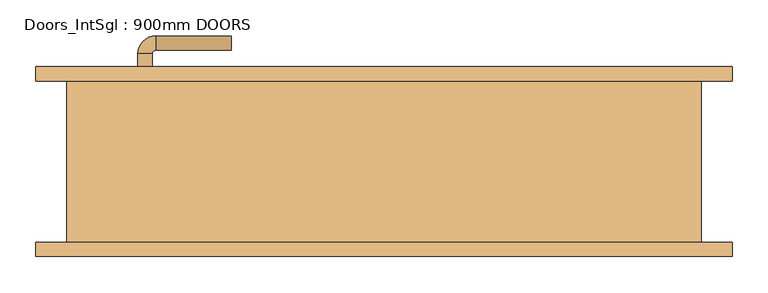
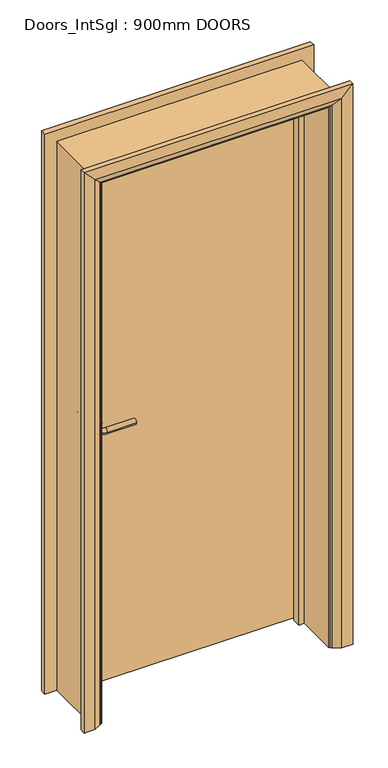
"""IFC4 building model written with IfcOpenShell, lengths in millimetres: door geometry, Doors_IntSgl : 900mm DOORS."""

from ifc_helpers import new_model, si_unit, point, frame, frame_2d, origin, place, context, project, spatial, polyline, circle_curve, ellipse_curve, trimmed, segment, composite_curve, outline, extrude, faceted_brep, source, transform, mapped, element, save
from ifc_brep_helpers import plane_surface, cylinder_surface, revolved_surface, advanced_brep


def doors_intsgl_900mm_doors_1c9cf9a6(model_context):
    return source(origin(), model_context, "Body", "SolidModel", [
        advanced_brep(
        [(-343.0, 66.5, 1000.0), (-323.0, 66.5, 1000.0), (-323.0, 36.5, 1000.0), (-343.0, 36.5, 1000.0), (-318.0, 31.5, 1000.0), (-318.0, 11.5, 1000.0), (-213.0, 11.5, 1000.0), (-213.0, 31.5, 1000.0)],
        [
            (0, 1, circle_curve(frame((-333.0, 66.5, 1000.0), z_axis=(0.0, 1.0, 0.0), x_axis=(1.0, 0.0, 0.0)), 10.0)),
            (1, 0, circle_curve(frame((-333.0, 66.5, 1000.0), z_axis=(0.0, 1.0, 0.0), x_axis=(1.0, 0.0, 0.0)), 10.0)),
            (1, 2),
            (2, 3, circle_curve(frame((-333.0, 36.5, 1000.0), z_axis=(0.0, 1.0, 0.0), x_axis=(1.0, 0.0, 0.0)), 10.0)),
            (3, 0),
            (3, 2, circle_curve(frame((-333.0, 36.5, 1000.0), z_axis=(0.0, 1.0, 0.0), x_axis=(1.0, 0.0, 0.0)), 10.0)),
            (4, 5, circle_curve(frame((-318.0, 21.5, 1000.0), z_axis=(-1.0, 0.0, 0.0), x_axis=(0.0, 1.0, 0.0)), 10.0)),
            (5, 3, circle_curve(frame((-318.0, 36.5, 1000.0), z_axis=(0.0, 0.0, -1.0), x_axis=(-1.0, 0.0, 0.0)), 25.0)),
            (2, 4, circle_curve(frame((-318.0, 36.5, 1000.0), z_axis=(0.0, 0.0, 1.0), x_axis=(-1.0, 0.0, 0.0)), 5.0)),
            (5, 4, circle_curve(frame((-318.0, 21.5, 1000.0), z_axis=(-1.0, 0.0, 0.0), x_axis=(0.0, 1.0, 0.0)), 10.0)),
            (6, 7, circle_curve(frame((-213.0, 21.5, 1000.0), z_axis=(1.0, 0.0, 0.0), x_axis=(0.0, 1.0, 0.0)), 10.0)),
            (7, 6, circle_curve(frame((-213.0, 21.5, 1000.0), z_axis=(1.0, 0.0, 0.0), x_axis=(0.0, 1.0, 0.0)), 10.0)),
            (4, 7),
            (6, 5),
        ],
        [
            plane_surface(frame((-333.0, 66.5, 1000.0), z_axis=(0.0, 1.0, 0.0), x_axis=(0.0, 0.0, 1.0))),
            cylinder_surface(frame((-333.0, 66.5, 1000.0), z_axis=(0.0, 1.0, 0.0), x_axis=(1.0, 0.0, 0.0)), 10.0),
            revolved_surface(trimmed(ellipse_curve(frame((-333.0, 36.5, 1000.0), z_axis=(0.0, -1.0, 0.0), x_axis=(1.0, 0.0, 0.0)), 10.0, 10.0), [point((-343.0, 36.5, 1000.0))], [point((-323.0, 36.5, 1000.0))], True, "CARTESIAN"), (-318.0, 36.5, 1000.0), (0.0, 0.0, -1.0)),
            revolved_surface(trimmed(ellipse_curve(frame((-333.0, 36.5, 1000.0), z_axis=(0.0, -1.0, 0.0), x_axis=(1.0, 0.0, 0.0)), 10.0, 10.0), [point((-323.0, 36.5, 1000.0))], [point((-343.0, 36.5, 1000.0))], True, "CARTESIAN"), (-318.0, 36.5, 1000.0), (0.0, 0.0, -1.0)),
            plane_surface(frame((-213.0, 21.5, 1000.0), z_axis=(1.0, 0.0, 0.0), x_axis=(0.0, 0.0, 1.0))),
            cylinder_surface(frame((-318.0, 21.5, 1000.0), z_axis=(-1.0, 0.0, 0.0), x_axis=(0.0, 1.0, 0.0)), 10.0),
        ],
        [
            (0, [[1, 2]]),
            (1, [[3, 4, 5, -2]]),
            (1, [[-5, 6, -3, -1]]),
            (2, [[7, 8, -4, 9]]),
            (3, [[10, -9, -6, -8]]),
            (4, [[11, 12]]),
            (5, [[13, -11, 14, -7]]),
            (5, [[-14, -12, -13, -10]]),
        ],
    ),
        extrude(outline(composite_curve([segment(trimmed(circle_curve(frame_2d((1000.0, -335.5)), 30.0), [point((1000.0, -365.5))], [point((1000.0, -305.5))], False, "CARTESIAN"), True, "CONTINUOUS"), segment(trimmed(circle_curve(frame_2d((1000.0, -335.5)), 30.0), [point((1000.0, -305.5))], [point((1000.0, -365.5))], False, "CARTESIAN"), True, "CONTINUOUS")], self_intersect=False)), frame((0.0, 66.5, 0.0), z_axis=(0.0, 1.0, 0.0), x_axis=(0.0, 0.0, 1.0)), (0.0, 0.0, 1.0), 8.0),
        advanced_brep(
        [(-343.0, 120.5, 1000.0), (-323.0, 120.5, 1000.0), (-343.0, 150.5, 1000.0), (-323.0, 150.5, 1000.0), (-318.0, 155.5, 1000.0), (-318.0, 175.5, 1000.0), (-213.0, 175.5, 1000.0), (-213.0, 155.5, 1000.0)],
        [
            (0, 1, circle_curve(frame((-333.0, 120.5, 1000.0), z_axis=(0.0, -1.0, 0.0), x_axis=(1.0, 0.0, 0.0)), 10.0)),
            (1, 0, circle_curve(frame((-333.0, 120.5, 1000.0), z_axis=(0.0, -1.0, 0.0), x_axis=(1.0, 0.0, 0.0)), 10.0)),
            (0, 2),
            (2, 3, circle_curve(frame((-333.0, 150.5, 1000.0), z_axis=(0.0, -1.0, 0.0), x_axis=(1.0, 0.0, 0.0)), 10.0)),
            (3, 1),
            (3, 2, circle_curve(frame((-333.0, 150.5, 1000.0), z_axis=(0.0, -1.0, 0.0), x_axis=(1.0, 0.0, 0.0)), 10.0)),
            (4, 3, circle_curve(frame((-318.0, 150.5, 1000.0), z_axis=(0.0, 0.0, 1.0), x_axis=(-1.0, 0.0, 0.0)), 5.0)),
            (2, 5, circle_curve(frame((-318.0, 150.5, 1000.0), z_axis=(0.0, 0.0, -1.0), x_axis=(-1.0, 0.0, 0.0)), 25.0)),
            (5, 4, circle_curve(frame((-318.0, 165.5, 1000.0), z_axis=(-1.0, 0.0, 0.0), x_axis=(0.0, -1.0, 0.0)), 10.0)),
            (4, 5, circle_curve(frame((-318.0, 165.5, 1000.0), z_axis=(-1.0, 0.0, 0.0), x_axis=(0.0, -1.0, 0.0)), 10.0)),
            (6, 7, circle_curve(frame((-213.0, 165.5, 1000.0), z_axis=(1.0, 0.0, 0.0), x_axis=(0.0, -1.0, 0.0)), 10.0)),
            (7, 6, circle_curve(frame((-213.0, 165.5, 1000.0), z_axis=(1.0, 0.0, 0.0), x_axis=(0.0, -1.0, 0.0)), 10.0)),
            (5, 6),
            (7, 4),
        ],
        [
            plane_surface(frame((-333.0, 120.5, 1000.0), z_axis=(0.0, -1.0, 0.0), x_axis=(0.0, 0.0, 1.0))),
            cylinder_surface(frame((-333.0, 120.5, 1000.0), z_axis=(0.0, -1.0, 0.0), x_axis=(1.0, 0.0, 0.0)), 10.0),
            revolved_surface(trimmed(ellipse_curve(frame((-333.0, 150.5, 1000.0), z_axis=(0.0, -1.0, 0.0), x_axis=(1.0, 0.0, 0.0)), 10.0, 10.0), [point((-343.0, 150.5, 1000.0))], [point((-323.0, 150.5, 1000.0))], True, "CARTESIAN"), (-318.0, 150.5, 1000.0), (0.0, 0.0, -1.0)),
            revolved_surface(trimmed(ellipse_curve(frame((-333.0, 150.5, 1000.0), z_axis=(0.0, -1.0, 0.0), x_axis=(1.0, 0.0, 0.0)), 10.0, 10.0), [point((-323.0, 150.5, 1000.0))], [point((-343.0, 150.5, 1000.0))], True, "CARTESIAN"), (-318.0, 150.5, 1000.0), (0.0, 0.0, -1.0)),
            plane_surface(frame((-213.0, 165.5, 1000.0), z_axis=(1.0, 0.0, 0.0), x_axis=(0.0, 0.0, 1.0))),
            cylinder_surface(frame((-318.0, 165.5, 1000.0), z_axis=(-1.0, 0.0, 0.0), x_axis=(0.0, -1.0, 0.0)), 10.0),
        ],
        [
            (0, [[1, 2]]),
            (1, [[-1, 3, 4, 5]]),
            (1, [[-2, -5, 6, -3]]),
            (2, [[7, -4, 8, 9]]),
            (3, [[-8, -6, -7, 10]]),
            (4, [[11, 12]]),
            (5, [[-9, 13, -12, 14]]),
            (5, [[-10, -14, -11, -13]]),
        ],
    ),
        extrude(outline(composite_curve([segment(trimmed(circle_curve(frame_2d((1000.0, -335.5)), 30.0), [point((1000.0, -365.5))], [point((1000.0, -305.5))], False, "CARTESIAN"), True, "CONTINUOUS"), segment(trimmed(circle_curve(frame_2d((1000.0, -335.5)), 30.0), [point((1000.0, -305.5))], [point((1000.0, -365.5))], False, "CARTESIAN"), True, "CONTINUOUS")], self_intersect=False)), frame((0.0, 112.5, 0.0), z_axis=(0.0, 1.0, 0.0), x_axis=(0.0, 0.0, 1.0)), (0.0, 0.0, 1.0), 8.0),
        extrude(outline(polyline([(408.0, 74.5), (-408.0, 74.5), (-408.0, 112.5), (408.0, 112.5), (408.0, 74.5)])), frame((0.0, 0.0, 8.0), z_axis=(0.0, 0.0, 1.0), x_axis=(1.0, 0.0, 0.0)), (0.0, 0.0, 1.0), 2050.0),
        faceted_brep([(-410.0, 112.5, 0.0), (-410.0, -112.5, 0.0), (-442.0, -112.5, 0.0), (-442.0, 112.5, 0.0), (-410.0, 112.5, 2060.0), (-410.0, -112.5, 2060.0), (-442.0, -112.5, 2092.0), (-442.0, 112.5, 2092.0), (410.0, 112.5, 0.0), (442.0, 112.5, 0.0), (442.0, -112.5, 0.0), (410.0, -112.5, 0.0), (410.0, 112.5, 2060.0), (442.0, 112.5, 2092.0), (442.0, -112.5, 2092.0), (410.0, -112.5, 2060.0)], [[[0, 1, 2, 3]], [[1, 0, 4, 5]], [[2, 1, 5, 6]], [[3, 2, 6, 7]], [[0, 3, 7, 4]], [[8, 9, 10, 11]], [[12, 13, 9, 8]], [[13, 14, 10, 9]], [[14, 15, 11, 10]], [[15, 12, 8, 11]], [[5, 4, 12, 15]], [[6, 5, 15, 14]], [[7, 6, 14, 13]], [[4, 7, 13, 12]]]),
        advanced_brep(
        [(-485.0, -132.5, 0.0), (-485.0, -112.5, 0.0), (-415.0, -112.5, 0.0), (-419.0, -118.5, 0.0), (-445.0, -132.5, 0.0), (-485.0, -132.5, 2135.0), (-485.0, -112.5, 2135.0), (-415.0, -112.5, 2065.0), (-419.0, -118.5, 2069.0), (-445.0, -132.5, 2095.0), (485.0, -132.5, 0.0), (445.0, -132.5, 0.0), (419.0, -118.5, 0.0), (415.0, -112.5, 0.0), (485.0, -112.5, 0.0), (485.0, -132.5, 2135.0), (445.0, -132.5, 2095.0), (419.0, -118.5, 2069.0), (415.0, -112.5, 2065.0), (485.0, -112.5, 2135.0)],
        [
            (0, 1),
            (1, 2),
            (2, 3, circle_curve(frame((-423.0, -111.5, 0.0), z_axis=(0.0, 0.0, -1.0), x_axis=(-1.0, 0.0, 0.0)), 8.0622577)),
            (3, 4),
            (4, 0),
            (0, 5),
            (5, 6),
            (6, 1),
            (6, 7),
            (7, 2),
            (7, 8, ellipse_curve(frame((-423.0, -111.5, 2073.0), z_axis=(-0.7071067811865475, 0.0, -0.7071067811865475), x_axis=(0.7071067811865474, 0.0, -0.7071067811865476)), 11.4017543, 8.0622577)),
            (8, 3),
            (8, 9),
            (9, 4),
            (9, 5),
            (10, 11),
            (11, 12),
            (12, 13, circle_curve(frame((423.0, -111.5, 0.0), z_axis=(0.0, 0.0, -1.0), x_axis=(1.0, 0.0, 0.0)), 8.0622577)),
            (13, 14),
            (14, 10),
            (15, 16),
            (16, 11),
            (10, 15),
            (16, 17),
            (17, 12),
            (17, 18, ellipse_curve(frame((423.0, -111.5, 2073.0), z_axis=(0.7071067811865475, 0.0, -0.7071067811865475), x_axis=(0.7071067811865474, 0.0, 0.7071067811865476)), 11.4017543, 8.0622577)),
            (18, 13),
            (18, 19),
            (19, 14),
            (19, 15),
            (5, 15),
            (19, 6),
            (18, 7),
            (17, 8),
            (16, 9),
        ],
        [
            plane_surface(frame((-415.0, -185.3010989, 0.0), z_axis=(0.0, 0.0, -1.0), x_axis=(1.0, 0.0, 0.0))),
            plane_surface(frame((-485.0, -132.5, 0.0), z_axis=(-1.0, 0.0, 0.0), x_axis=(0.0, 0.0, 1.0))),
            plane_surface(frame((-485.0, -112.5, 0.0), z_axis=(0.0, 1.0, 0.0), x_axis=(0.0, 0.0, 1.0))),
            cylinder_surface(frame((-423.0, -111.5, 0.0), z_axis=(0.0, 0.0, -1.0), x_axis=(-1.0, 0.0, 0.0)), 8.0622577),
            plane_surface(frame((-419.0, -118.5, 0.0), z_axis=(0.4740998230350183, -0.8804710999221749, 0.0), x_axis=(0.0, 0.0, 1.0))),
            plane_surface(frame((-445.0, -132.5, 0.0), z_axis=(0.0, -1.0, 0.0), x_axis=(0.0, 0.0, 1.0))),
            plane_surface(frame((415.0, -185.3010989, 0.0), z_axis=(0.0, 0.0, -1.0), x_axis=(-1.0, 0.0, 0.0))),
            plane_surface(frame((445.0, -132.5, 2095.0), z_axis=(0.0, -1.0, 0.0), x_axis=(0.0, 0.0, -1.0))),
            plane_surface(frame((419.0, -118.5, 2069.0), z_axis=(-0.4740998230350183, -0.8804710999221749, 0.0), x_axis=(0.0, 0.0, -1.0))),
            cylinder_surface(frame((423.0, -111.5, 2065.0), z_axis=(0.0, 0.0, 1.0), x_axis=(1.0, 0.0, 0.0)), 8.0622577),
            plane_surface(frame((485.0, -112.5, 2135.0), z_axis=(0.0, 1.0, 0.0), x_axis=(0.0, 0.0, -1.0))),
            plane_surface(frame((485.0, -132.5, 2135.0), z_axis=(1.0, 0.0, 0.0), x_axis=(0.0, 0.0, -1.0))),
            plane_surface(frame((-485.0, -132.5, 2135.0), z_axis=(0.0, 0.0, 1.0), x_axis=(1.0, 0.0, 0.0))),
            plane_surface(frame((-485.0, -112.5, 2135.0), z_axis=(0.0, 1.0, 0.0), x_axis=(1.0, 0.0, 0.0))),
            cylinder_surface(frame((-415.0, -111.5, 2073.0), z_axis=(-1.0, 0.0, 0.0), x_axis=(0.0, 0.0, 1.0)), 8.0622577),
            plane_surface(frame((-419.0, -118.5, 2069.0), z_axis=(0.0, -0.8804710999221749, -0.4740998230350183), x_axis=(1.0, 0.0, 0.0))),
            plane_surface(frame((-445.0, -132.5, 2095.0), z_axis=(0.0, -1.0, 0.0), x_axis=(1.0, 0.0, 0.0))),
        ],
        [
            (0, [[1, 2, 3, 4, 5]]),
            (1, [[-1, 6, 7, 8]]),
            (2, [[-2, -8, 9, 10]]),
            (3, [[-3, -10, 11, 12]]),
            (4, [[-4, -12, 13, 14]]),
            (5, [[-5, -14, 15, -6]]),
            (6, [[16, 17, 18, 19, 20]]),
            (7, [[21, 22, -16, 23]]),
            (8, [[24, 25, -17, -22]]),
            (9, [[26, 27, -18, -25]]),
            (10, [[28, 29, -19, -27]]),
            (11, [[30, -23, -20, -29]]),
            (12, [[-7, 31, -30, 32]]),
            (13, [[-9, -32, -28, 33]]),
            (14, [[-11, -33, -26, 34]]),
            (15, [[-13, -34, -24, 35]]),
            (16, [[-15, -35, -21, -31]]),
        ],
    ),
        extrude(outline(polyline([(0.0, -410.0), (0.0, -391.0), (2041.0, -391.0), (2041.0, 391.0), (0.0, 391.0), (0.0, 410.0), (2060.0, 410.0), (2060.0, -410.0), (0.0, -410.0)])), frame((0.0, 40.5, 0.0), z_axis=(0.0, 1.0, 0.0), x_axis=(0.0, 0.0, 1.0)), (0.0, 0.0, 1.0), 32.0),
        advanced_brep(
        [(485.0, 132.5, 0.0), (485.0, 112.5, 0.0), (415.0, 112.5, 0.0), (419.0, 118.5, 0.0), (445.0, 132.5, 0.0), (485.0, 132.5, 2135.0), (485.0, 112.5, 2135.0), (-485.0, 112.5, 2135.0), (-485.0, 112.5, 0.0), (-415.0, 112.5, 0.0), (-415.0, 112.5, 2065.0), (415.0, 112.5, 2065.0), (419.0, 118.5, 2069.0), (445.0, 132.5, 2095.0), (-445.0, 132.5, 2095.0), (-445.0, 132.5, 0.0), (-485.0, 132.5, 0.0), (-485.0, 132.5, 2135.0), (-419.0, 118.5, 0.0), (-419.0, 118.5, 2069.0)],
        [
            (0, 1),
            (1, 2),
            (2, 3, circle_curve(frame((423.0, 111.5, 0.0), z_axis=(0.0, 0.0, -1.0), x_axis=(1.0, 0.0, 0.0)), 8.0622577)),
            (3, 4),
            (4, 0),
            (0, 5),
            (5, 6),
            (6, 1),
            (6, 7),
            (7, 8),
            (8, 9),
            (9, 10),
            (10, 11),
            (11, 2),
            (11, 12, ellipse_curve(frame((423.0, 111.5, 2073.0), z_axis=(0.7071067811865475, 0.0, -0.7071067811865475), x_axis=(-0.7071067811865474, 0.0, -0.7071067811865476)), 11.4017543, 8.0622577)),
            (12, 3),
            (12, 13),
            (13, 4),
            (13, 14),
            (14, 15),
            (15, 16),
            (16, 17),
            (17, 5),
            (7, 17),
            (16, 8),
            (15, 18),
            (18, 9, circle_curve(frame((-423.0, 111.5, 0.0), z_axis=(0.0, 0.0, -1.0), x_axis=(-1.0, 0.0, 0.0)), 8.0622577)),
            (19, 10, ellipse_curve(frame((-423.0, 111.5, 2073.0), z_axis=(-0.7071067811865475, 0.0, -0.7071067811865475), x_axis=(-0.7071067811865474, 0.0, 0.7071067811865476)), 11.4017543, 8.0622577)),
            (18, 19),
            (14, 19),
            (19, 12),
        ],
        [
            plane_surface(frame((415.0, 112.5, 0.0), z_axis=(0.0, 0.0, -1.0), x_axis=(0.0, -1.0, 0.0))),
            plane_surface(frame((485.0, 132.5, 0.0), z_axis=(1.0, 0.0, 0.0), x_axis=(0.0, 0.0, 1.0))),
            plane_surface(frame((485.0, 112.5, 0.0), z_axis=(0.0, -1.0, 0.0), x_axis=(0.0, 0.0, 1.0))),
            cylinder_surface(frame((423.0, 111.5, 0.0), z_axis=(0.0, 0.0, -1.0), x_axis=(1.0, 0.0, 0.0)), 8.0622577),
            plane_surface(frame((419.0, 118.5, 0.0), z_axis=(-0.4740998230350126, 0.880471099922178, 0.0), x_axis=(0.0, 0.0, 1.0))),
            plane_surface(frame((445.0, 132.5, 0.0), z_axis=(0.0, 1.0, 0.0), x_axis=(0.0, 0.0, 1.0))),
            plane_surface(frame((-485.0, 132.5, 2135.0), z_axis=(-1.0, 0.0, 0.0), x_axis=(0.0, 0.0, -1.0))),
            plane_surface(frame((-415.0, 112.5, 0.0), z_axis=(0.0, 0.0, -1.0), x_axis=(0.0, -1.0, 0.0))),
            cylinder_surface(frame((-423.0, 111.5, 2065.0), z_axis=(0.0, 0.0, 1.0), x_axis=(-1.0, 0.0, 0.0)), 8.0622577),
            plane_surface(frame((-419.0, 118.5, 2069.0), z_axis=(0.47409982303501824, 0.8804710999221749, 0.0), x_axis=(0.0, 0.0, -1.0))),
            plane_surface(frame((485.0, 132.5, 2135.0), z_axis=(0.0, 0.0, 1.0), x_axis=(-1.0, 0.0, 0.0))),
            cylinder_surface(frame((415.0, 111.5, 2073.0), z_axis=(1.0, 0.0, 0.0), x_axis=(0.0, 0.0, 1.0)), 8.0622577),
            plane_surface(frame((419.0, 118.5, 2069.0), z_axis=(0.0, 0.8804710999221764, -0.4740998230350154), x_axis=(-1.0, 0.0, 0.0))),
        ],
        [
            (0, [[1, 2, 3, 4, 5]]),
            (1, [[-1, 6, 7, 8]]),
            (2, [[-2, -8, 9, 10, 11, 12, 13, 14]]),
            (3, [[-3, -14, 15, 16]]),
            (4, [[-4, -16, 17, 18]]),
            (5, [[-5, -18, 19, 20, 21, 22, 23, -6]]),
            (6, [[24, -22, 25, -10]]),
            (7, [[-21, 26, 27, -11, -25]]),
            (8, [[28, -12, -27, 29]]),
            (9, [[30, -29, -26, -20]]),
            (10, [[-7, -23, -24, -9]]),
            (11, [[-15, -13, -28, 31]]),
            (12, [[-17, -31, -30, -19]]),
        ],
    ),
    ])


if __name__ == "__main__":
    model = new_model("IFC4")
    model_context = context("Model", 3, world=origin())
    ifc_project = project(units=[si_unit("LENGTHUNIT", "METRE", prefix="MILLI")], contexts=[model_context])
    site = spatial("IfcSite", under=ifc_project)
    building = spatial("IfcBuilding", under=site)
    placement = place(None, origin())
    doors_intsgl_900mm_doors_shape = doors_intsgl_900mm_doors_1c9cf9a6(model_context)
    element("IfcDoor", 1, ObjectType="Doors_IntSgl : 900mm DOORS", at=placement, inside=building, context=model_context, shape_type="MappedRepresentation", body=[
        mapped(doors_intsgl_900mm_doors_shape, transform((0.0, 0.0, 0.0), x_axis=(1.0, 0.0, 0.0), y_axis=(0.0, 1.0, 0.0), z_axis=(0.0, 0.0, 1.0))),
    ])
    save(model, "model.ifc")

# Revit data of these elements
# Type "Doors_IntSgl : 900mm DOORS"
#   Type Mark = "46"
#   Type Comments = "Internal Single"
#   Operation = "SingleSwingRight"
#   Manufacturer = "Revit"
#   Keynote = "L20"
#   Description = "Internal Single Door"
#   Analytic Construction = "Metal"
#   UnderCut = 8 mm
#   Tolerance = 2 mm
#   Thickness = 38 mm
#   Thermal Resistance (R) = 0.270117 (m²·K)/W
#   Structural Tolerance = 8 mm
#   StopDepth = 32 mm
#   Stop Thickness = 19 mm
#   Rough Width = 900 mm
#   Rough Height = 2100 mm
#   Height to Top Lock Rail = 1000 mm
#   Heat Transfer Coefficient (U) = 3.7021 W/(m²·K)
#   Handle Z Distance = 1000 mm
#   Handle X Distance = 75 mm
#   Frame Thickness = 32 mm
#   Door Panel Width = 816 mm
#   Door Panel Thickness = 38 mm
#   Door Panel Offset = 0 mm
#   Height = 2100 mm
#   Width = 900 mm
#   Door Panel Height = 2050 mm
#   Architrave Setback = 5 mm
#   Vis - Ironmongery = yes
#   Define Thermal Properties by = 1
#   Material Ironmongery = Door - Handle
#   Material Frame = Door - Frame/Mullion (1)
#   Material Door = Door - Panel
#   Material Architrave = Door - Architrave
#   Visual Light Transmittance = 0
#   Solar Heat Gain Coefficient = 0
#   Function = (empty or 0)
#   Wall Closure = (empty or 0)
# Element 1 (IfcDoor, "Doors_IntSgl : 900mm DOORS")
#   Materials on its faces: "Door - Architrave", "Door - Handle", "Door - Frame/Mullion (1)", "Door - Panel"
# Materials
#   "Door - Handle": colour RGB 0 0 0, transparency 0, Cost = 0
#   "Door - Frame/Mullion (1)": class "Wood", colour RGB 212 179 113, transparency 0, Keynote = "L20", Cost = 0
#   "Door - Panel": class "Wood", colour RGB 210 159 95, transparency 0, Cost = 0
#   "Door - Architrave": class "Wood", colour RGB 154 90 5, transparency 0, Keynote = "P20", Cost = 0
